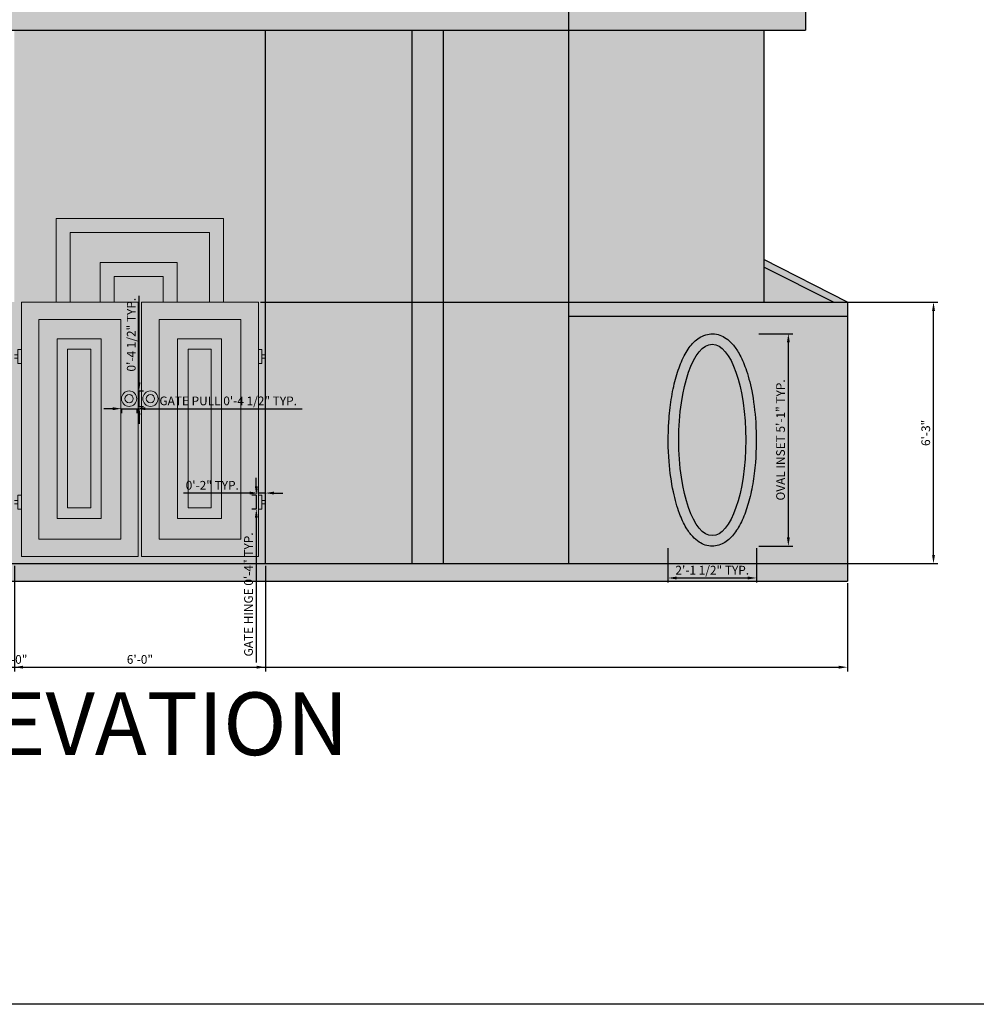
# Model space of a CAD drawing. Units: inches. Extents: x 2169 to 10664, y 1669 to 6352.
# Tile 14 of 17: x 9778 to 10052, y 5159 to 5441. Entities that reach past the tile are written whole.
import ezdxf

# ---------------------------------------------------------------- set-up
doc = ezdxf.new("R2010")
doc.units = ezdxf.units.IN
for name, color, linetype, lineweight in [('A-ANNO-DIMS', 3, 'Continuous', 18), ('A-ANNO-TITL', 3, 'Continuous', 25), ('A-ANNO-TTLB', 7, 'Continuous', 25), ('A-ELEV', 7, 'Continuous', 25), ('A-ELEV-CONC-PATT', 85, 'Continuous', 13), ('A-ELEV-GATE', 7, 'Continuous', 18), ('A-ELEV-GATE-PATT', 252, 'Continuous', 13), ('A-ELEV-OPEN', 7, 'Continuous', 18), ('A-ELEV-OPEN-PATT', 9, 'Continuous', 13), ('A-ELEV-PATT', 253, 'Continuous', 13)]:
    doc.layers.add(name, color=color, linetype=linetype, lineweight=lineweight)
doc.styles.get("Standard").update_dxf_attribs({"font": 'arial.ttf'})
doc.dimstyles.new('ISO-25', dxfattribs={"dimtxt": 2.5, "dimasz": 2.5, "dimexe": 1.25, "dimexo": 0.625, "dimtad": 1, "dimdec": 0, "dimlunit": 3, "dimtxsty": 'Standard', "dimcen": 2.5, "dimadec": 0, "dimazin": 0, "dimtfac": 1, "dimtdec": 0, "dimtmove": 0, "dimatfit": 3, "dimfxl": 1, "dimarcsym": 0})

# ---------------------------------------------------------------- blocks, each defined once
blk = doc.blocks.new('GATE-HINGE-3')
for p, q in [((2, 4), (1, 4)), ((1, 4), (1, 0)), ((1, 2.5), (0, 2.5)), ((1, 1.5), (0, 1.5)), ((2, 0), (1, 0))]:
    blk.add_line(p, q)
blk = doc.blocks.new('GATE-PULL-ROUND')
for radius in [2.2, 1.2]:
    blk.add_circle((2.21, 2.21), radius)
blk = doc.blocks.new('FACADE-OVAL-INSET')
blk.add_ellipse((12.63, 30.44), major_axis=(0, -27.44), ratio=0.350877)
blk.add_open_spline([(12.63, 0), (13.28, 0), (13.93, 0.1), (15.16, 0.48), (15.73, 0.75), (16.8, 1.42), (17.29, 1.81), (18.2, 2.68), (18.63, 3.16), (19.86, 4.78), (20.59, 6.05), (21.9, 8.93), (22.47, 10.53), (23.47, 14), (23.89, 15.87), (24.57, 19.81), (24.82, 21.88), (25.3, 27.78), (25.34, 31.73), (24.89, 38.68), (24.51, 41.73), (23.49, 46.87), (22.91, 49.03), (21.66, 52.55), (21.03, 53.98), (19.74, 56.25), (19.12, 57.16), (17.87, 58.57), (17.27, 59.12), (16.05, 59.96), (15.45, 60.28), (14.17, 60.73), (13.48, 60.86), (12.09, 60.9), (11.4, 60.8), (10.08, 60.4), (9.47, 60.11), (8.34, 59.39), (7.83, 58.96), (6.87, 58.01), (6.43, 57.49), (5.17, 55.76), (4.44, 54.41), (3.14, 51.39), (2.57, 49.71), (1.59, 46.07), (1.19, 44.12), (0.55, 40.02), (0.31, 37.87), (-0.08, 31.9), (-0.06, 28), (0.48, 21.2), (0.89, 18.26), (1.95, 13.31), (2.54, 11.23), (3.8, 7.86), (4.43, 6.5), (5.71, 4.33), (6.34, 3.47), (7.58, 2.13), (8.18, 1.61), (9.39, 0.82), (9.99, 0.52), (11.27, 0.11), (11.95, 0), (12.63, 0)], degree=3, knots=[0, 0, 0, 0, 0.107478, 0.107478, 0.214955, 0.214955, 0.322433, 0.322433, 0.429911, 0.429911, 0.658113, 0.658113, 0.886316, 0.886316, 1.114519, 1.114519, 1.342721, 1.342721, 1.750863, 1.750863, 2.0857, 2.0857, 2.362812, 2.362812, 2.586848, 2.586848, 2.764909, 2.764909, 2.903641, 2.903641, 3.018249, 3.018249, 3.132858, 3.132858, 3.247466, 3.247466, 3.362074, 3.362074, 3.476683, 3.476683, 3.591291, 3.591291, 3.82536, 3.82536, 4.059428, 4.059428, 4.293497, 4.293497, 4.527566, 4.527566, 4.931556, 4.931556, 5.258929, 5.258929, 5.530471, 5.530471, 5.749212, 5.749212, 5.922827, 5.922827, 6.058126, 6.058126, 6.171203, 6.171203, 6.283185, 6.283185, 6.283185, 6.283185])
blk = doc.blocks.new('*D67')
at = {"layer": 'A-ANNO-DIMS', "color": 0, "lineweight": -2, "transparency": 16777216}
for p, q in [((9804.65, 5329.75), (9802.15, 5329.75)), ((9807.15, 5329.78), (9807.15, 5328.5)), ((9807.15, 5329.75), (9811.56, 5329.75)), ((9811.56, 5329.78), (9811.56, 5328.5)), ((9814.06, 5329.75), (9859.02, 5329.75))]:
    blk.add_line(p, q, dxfattribs=at)
at = {"layer": 'A-ANNO-DIMS', "color": 0, "transparency": 16777216}
for points in [[(9804.65, 5330.16), (9804.65, 5329.33), (9807.15, 5329.75)], [(9814.06, 5330.16), (9814.06, 5329.33), (9811.56, 5329.75)]]:
    blk.add_solid(points, dxfattribs=at)
at = {"layer": 'Defpoints', "color": 0, "transparency": 16777216}
for p in [(9807.15, 5330.41), (9811.56, 5330.41), (9811.56, 5329.75)]:
    blk.add_point(p, dxfattribs=at)
at = {"layer": 'A-ANNO-DIMS', "color": 0, "transparency": 16777216, "insert": (9837.79, 5331.66), "char_height": 2.5, "attachment_point": 5}
blk.add_mtext('GATE PULL 0\'-4 1/2" TYP.', dxfattribs=at)
blk = doc.blocks.new('*D68')
at = {"layer": 'A-ANNO-DIMS', "color": 0, "lineweight": -2, "transparency": 16777216}
for p, q in [((9812.22, 5337.32), (9812.22, 5362.13)), ((9812.18, 5334.82), (9813.47, 5334.82)), ((9812.22, 5330.41), (9812.22, 5334.82)), ((9812.18, 5330.41), (9813.47, 5330.41)), ((9812.22, 5327.91), (9812.22, 5325.41))]:
    blk.add_line(p, q, dxfattribs=at)
at = {"layer": 'A-ANNO-DIMS', "color": 0, "transparency": 16777216}
for points in [[(9811.8, 5337.32), (9812.63, 5337.32), (9812.22, 5334.82)], [(9811.8, 5327.91), (9812.63, 5327.91), (9812.22, 5330.41)]]:
    blk.add_solid(points, dxfattribs=at)
at = {"layer": 'Defpoints', "color": 0, "transparency": 16777216}
for p in [(9811.56, 5334.82), (9812.22, 5334.82), (9811.56, 5330.41)]:
    blk.add_point(p, dxfattribs=at)
at = {"layer": 'A-ANNO-DIMS', "color": 0, "transparency": 16777216, "insert": (9810.3, 5350.97), "char_height": 2.5, "attachment_point": 5, "rotation": 90}
blk.add_mtext('0\'-4 1/2" TYP.', dxfattribs=at)
blk = doc.blocks.new('*D71')
at = {"layer": 'A-ANNO-DIMS', "color": 0, "lineweight": -2, "transparency": 16777216}
for p, q in [((9845.86, 5307.45), (9845.86, 5309.95)), ((9845.84, 5304.95), (9844.61, 5304.95)), ((9845.86, 5304.95), (9845.86, 5300.95)), ((9845.84, 5300.95), (9844.61, 5300.95)), ((9845.86, 5298.45), (9845.86, 5256.99))]:
    blk.add_line(p, q, dxfattribs=at)
at = {"layer": 'A-ANNO-DIMS', "color": 0, "transparency": 16777216}
for points in [[(9845.45, 5307.45), (9846.28, 5307.45), (9845.86, 5304.95)], [(9845.45, 5298.45), (9846.28, 5298.45), (9845.86, 5300.95)]]:
    blk.add_solid(points, dxfattribs=at)
at = {"layer": 'Defpoints', "color": 0, "transparency": 16777216}
for p in [(9846.46, 5304.95), (9845.86, 5300.95), (9846.46, 5300.95)]:
    blk.add_point(p, dxfattribs=at)
at = {"layer": 'A-ANNO-DIMS', "color": 0, "transparency": 16777216, "insert": (9843.94, 5276.47), "char_height": 2.5, "attachment_point": 5, "rotation": 90}
blk.add_mtext('GATE HINGE 0\'-4" TYP.', dxfattribs=at)
blk = doc.blocks.new('*D72')
at = {"layer": 'A-ANNO-DIMS', "color": 0, "lineweight": -2, "transparency": 16777216}
for p, q in [((9846.46, 5305.57), (9846.46, 5306.8)), ((9848.46, 5305.57), (9848.46, 5306.8)), ((9843.96, 5305.55), (9824.97, 5305.55)), ((9848.46, 5305.55), (9846.46, 5305.55)), ((9850.96, 5305.55), (9853.46, 5305.55))]:
    blk.add_line(p, q, dxfattribs=at)
at = {"layer": 'A-ANNO-DIMS', "color": 0, "transparency": 16777216}
for points in [[(9843.96, 5305.97), (9843.96, 5305.13), (9846.46, 5305.55)], [(9850.96, 5305.97), (9850.96, 5305.13), (9848.46, 5305.55)]]:
    blk.add_solid(points, dxfattribs=at)
at = {"layer": 'Defpoints', "color": 0, "transparency": 16777216}
for p in [(9846.46, 5305.55), (9846.46, 5304.95), (9848.46, 5304.95)]:
    blk.add_point(p, dxfattribs=at)
at = {"layer": 'A-ANNO-DIMS', "color": 0, "transparency": 16777216, "insert": (9833.22, 5307.45), "char_height": 2.5, "attachment_point": 5}
blk.add_mtext('0\'-2" TYP.', dxfattribs=at)
blk = doc.blocks.new('*D73')
at = {"layer": 'A-ANNO-DIMS', "color": 0, "lineweight": -2, "transparency": 16777216}
for p, q in [((9990.01, 5351.23), (9999.77, 5351.23)), ((9998.52, 5292.83), (9998.52, 5348.73)), ((9990.01, 5290.33), (9999.77, 5290.33))]:
    blk.add_line(p, q, dxfattribs=at)
at = {"layer": 'A-ANNO-DIMS', "color": 0, "transparency": 16777216}
for points in [[(9998.1, 5348.73), (9998.94, 5348.73), (9998.52, 5351.23)], [(9998.1, 5292.83), (9998.94, 5292.83), (9998.52, 5290.33)]]:
    blk.add_solid(points, dxfattribs=at)
at = {"layer": 'Defpoints', "color": 0, "transparency": 16777216}
for p in [(9989.38, 5351.23), (9998.52, 5351.23), (9989.38, 5290.33)]:
    blk.add_point(p, dxfattribs=at)
at = {"layer": 'A-ANNO-DIMS', "color": 0, "transparency": 16777216, "insert": (9996.6, 5320.78), "char_height": 2.5, "attachment_point": 5, "rotation": 90}
blk.add_mtext('OVAL INSET 5\'-1" TYP.', dxfattribs=at)
blk = doc.blocks.new('*D74')
at = {"layer": 'A-ANNO-DIMS', "color": 0, "lineweight": -2, "transparency": 16777216}
for p, q in [((9963.97, 5289.7), (9963.97, 5279.94)), ((9989.38, 5289.7), (9989.38, 5279.94)), ((9966.47, 5281.19), (9986.88, 5281.19))]:
    blk.add_line(p, q, dxfattribs=at)
at = {"layer": 'A-ANNO-DIMS', "color": 0, "transparency": 16777216}
for points in [[(9966.47, 5281.61), (9966.47, 5280.78), (9963.97, 5281.19)], [(9986.88, 5281.61), (9986.88, 5280.78), (9989.38, 5281.19)]]:
    blk.add_solid(points, dxfattribs=at)
at = {"layer": 'Defpoints', "color": 0, "transparency": 16777216}
for p in [(9963.97, 5290.33), (9989.38, 5290.33), (9989.38, 5281.19)]:
    blk.add_point(p, dxfattribs=at)
at = {"layer": 'A-ANNO-DIMS', "color": 0, "transparency": 16777216, "insert": (9976.68, 5283.11), "char_height": 2.5, "attachment_point": 5}
blk.add_mtext('2\'-1 1/2" TYP.', dxfattribs=at)
blk = doc.blocks.new('*D117')
at = {"layer": 'A-ANNO-DIMS', "color": 0, "lineweight": -2, "transparency": 16777216}
for p, q in [((9535.46, 5279.69), (9535.46, 5254.36)), ((10015.46, 5279.69), (10015.46, 5254.36)), ((9537.96, 5255.61), (10012.96, 5255.61))]:
    blk.add_line(p, q, dxfattribs=at)
at = {"layer": 'A-ANNO-DIMS', "color": 0, "transparency": 16777216}
for points in [[(9537.96, 5256.03), (9537.96, 5255.19), (9535.46, 5255.61)], [(10012.96, 5256.03), (10012.96, 5255.19), (10015.46, 5255.61)]]:
    blk.add_solid(points, dxfattribs=at)
at = {"layer": 'Defpoints', "color": 0, "transparency": 16777216}
for p in [(9535.46, 5280.31), (10015.46, 5280.31), (10015.46, 5255.61)]:
    blk.add_point(p, dxfattribs=at)
at = {"layer": 'A-ANNO-DIMS', "color": 0, "transparency": 16777216, "insert": (9775.46, 5257.51), "char_height": 2.5, "attachment_point": 5}
blk.add_mtext('40\'-0"', dxfattribs=at)
blk = doc.blocks.new('*D124')
at = {"layer": 'A-ANNO-DIMS', "color": 0, "lineweight": -2, "transparency": 16777216}
for p, q in [((9776.46, 5284.69), (9776.46, 5254.36)), ((9848.46, 5284.69), (9848.46, 5254.36)), ((9778.96, 5255.61), (9845.96, 5255.61))]:
    blk.add_line(p, q, dxfattribs=at)
at = {"layer": 'A-ANNO-DIMS', "color": 0, "transparency": 16777216}
for points in [[(9778.96, 5256.03), (9778.96, 5255.19), (9776.46, 5255.61)], [(9845.96, 5256.03), (9845.96, 5255.19), (9848.46, 5255.61)]]:
    blk.add_solid(points, dxfattribs=at)
at = {"layer": 'Defpoints', "color": 0, "transparency": 16777216}
for p in [(9776.46, 5285.31), (9848.46, 5285.31), (9848.46, 5255.61)]:
    blk.add_point(p, dxfattribs=at)
at = {"layer": 'A-ANNO-DIMS', "color": 0, "transparency": 16777216, "insert": (9812.46, 5257.51), "char_height": 2.5, "attachment_point": 5}
blk.add_mtext('6\'-0"', dxfattribs=at)
blk = doc.blocks.new('*D125')
at = {"layer": 'A-ANNO-DIMS', "color": 0, "lineweight": -2, "transparency": 16777216}
for p, q in [((9847.09, 5360.31), (10041.41, 5360.31)), ((10040.16, 5287.81), (10040.16, 5357.81)), ((9849.09, 5285.31), (10041.41, 5285.31))]:
    blk.add_line(p, q, dxfattribs=at)
at = {"layer": 'A-ANNO-DIMS', "color": 0, "transparency": 16777216}
for points in [[(10039.75, 5357.81), (10040.58, 5357.81), (10040.16, 5360.31)], [(10039.75, 5287.81), (10040.58, 5287.81), (10040.16, 5285.31)]]:
    blk.add_solid(points, dxfattribs=at)
at = {"layer": 'Defpoints', "color": 0, "transparency": 16777216}
for p in [(9846.46, 5360.31), (10040.16, 5360.31), (9848.46, 5285.31)]:
    blk.add_point(p, dxfattribs=at)
at = {"layer": 'A-ANNO-DIMS', "color": 0, "transparency": 16777216, "insert": (10038.26, 5322.81), "char_height": 2.5, "attachment_point": 5, "rotation": 90}
blk.add_mtext('6\'-3"', dxfattribs=at)

msp = doc.modelspace()

# ---------------------------------------------------------------- hatches: boundary and pattern name
at = {"layer": 'A-ELEV-CONC-PATT'}
h = msp.add_hatch(dxfattribs=at)
h.set_pattern_fill('AR-CONC', color=256, scale=0.02)
h.paths.add_polyline_path([(9899.46, 5522.31), (9776.46, 5522.31), (9776.46, 5513.31), (9890.46, 5513.31), (9890.46, 5444.31), (9899.46, 5444.31)])
h.paths.add_polyline_path([(9899.46, 5438.31), (9890.46, 5438.31), (9890.46, 5285.31), (9899.46, 5285.31)])
at = {"layer": 'A-ELEV-GATE-PATT'}
h = msp.add_hatch(color=256, dxfattribs=at)
h.dxf.hatch_style = 1
h.paths.add_polyline_path([(9778.46, 5346.71), (9777.46, 5346.71), (9777.46, 5342.71), (9778.46, 5342.71)])
h.paths.add_polyline_path([(9777.46, 5345.21), (9776.46, 5345.21), (9776.46, 5344.21), (9777.46, 5344.21)])
h.paths.add_polyline_path([(9848.46, 5345.21), (9847.46, 5345.21), (9847.46, 5344.21), (9848.46, 5344.21)])
h.paths.add_polyline_path([(9847.46, 5346.71), (9846.46, 5346.71), (9846.46, 5342.71), (9847.46, 5342.71)])
h.paths.add_polyline_path([(9847.46, 5304.95), (9846.46, 5304.95), (9846.46, 5300.95), (9847.46, 5300.95)])
h.paths.add_polyline_path([(9848.46, 5303.45), (9847.46, 5303.45), (9847.46, 5302.45), (9848.46, 5302.45)])
h.paths.add_polyline_path([(9778.46, 5304.95), (9777.46, 5304.95), (9777.46, 5300.95), (9778.46, 5300.95)])
h.paths.add_polyline_path([(9777.46, 5303.45), (9776.46, 5303.45), (9776.46, 5302.45), (9777.46, 5302.45)])
h.paths.add_polyline_path([(9811.96, 5360.31), (9778.46, 5360.31), (9778.46, 5287.31), (9811.96, 5287.31)])
h.paths.add_polyline_path([(9783.46, 5355.31), (9806.96, 5355.31), (9806.96, 5292.31), (9783.46, 5292.31)], flags=16)
h.paths.add_polyline_path([(9788.71, 5349.82), (9801.33, 5349.82), (9801.33, 5298.27), (9788.71, 5298.27)], flags=0)
h.paths.add_polyline_path([(9791.71, 5346.82), (9798.33, 5346.82), (9798.33, 5301.27), (9791.71, 5301.27)], flags=0)
h.paths.add_polyline_path([(9807.16, 5332.61, -1), (9811.54, 5332.61, -1)], flags=16)
h.paths.add_polyline_path([(9808.16, 5332.61, -1), (9810.54, 5332.61, -1)], flags=0)
h.paths.add_polyline_path([(9846.46, 5360.31), (9812.96, 5360.31), (9812.96, 5287.31), (9846.46, 5287.31)])
h.paths.add_polyline_path([(9817.96, 5355.31), (9841.46, 5355.31), (9841.46, 5292.31), (9817.96, 5292.31)], flags=16)
h.paths.add_polyline_path([(9823.29, 5349.82), (9835.91, 5349.82), (9835.91, 5298.27), (9823.29, 5298.27)], flags=0)
h.paths.add_polyline_path([(9826.29, 5346.82), (9832.91, 5346.82), (9832.91, 5301.27), (9826.29, 5301.27)], flags=0)
h.paths.add_polyline_path([(9813.3, 5332.61, -1), (9817.67, 5332.61, -1)], flags=16)
h.paths.add_polyline_path([(9814.3, 5332.61, -1), (9816.67, 5332.61, -1)], flags=0)
h.paths.add_polyline_path([(9801.33, 5349.82), (9788.71, 5349.82), (9788.71, 5298.27), (9801.33, 5298.27)], flags=0)
h = msp.add_hatch(color=256, dxfattribs=at)
h.dxf.hatch_style = 1
h.paths.add_polyline_path([(9806.96, 5355.31), (9783.46, 5355.31), (9783.46, 5292.31), (9806.96, 5292.31)])
h.paths.add_polyline_path([(9788.71, 5349.82), (9801.33, 5349.82), (9801.33, 5298.27), (9788.71, 5298.27)], flags=16)
h.paths.add_polyline_path([(9791.71, 5346.82), (9798.33, 5346.82), (9798.33, 5301.27), (9791.71, 5301.27)], flags=0)
h.paths.add_polyline_path([(9841.46, 5355.31), (9817.96, 5355.31), (9817.96, 5292.31), (9841.46, 5292.31)])
h.paths.add_polyline_path([(9823.29, 5349.82), (9835.91, 5349.82), (9835.91, 5298.27), (9823.29, 5298.27)], flags=16)
h.paths.add_polyline_path([(9826.29, 5346.82), (9832.91, 5346.82), (9832.91, 5301.27), (9826.29, 5301.27)], flags=0)
h = msp.add_hatch(color=256, dxfattribs=at)
h.dxf.hatch_style = 1
h.paths.add_polyline_path([(9801.33, 5349.82), (9788.71, 5349.82), (9788.71, 5298.27), (9801.33, 5298.27)])
h.paths.add_polyline_path([(9791.71, 5346.82), (9798.33, 5346.82), (9798.33, 5301.27), (9791.71, 5301.27)], flags=16)
h.paths.add_polyline_path([(9835.91, 5349.82), (9823.29, 5349.82), (9823.29, 5298.27), (9835.91, 5298.27)])
h.paths.add_polyline_path([(9826.29, 5346.82), (9832.91, 5346.82), (9832.91, 5301.27), (9826.29, 5301.27)], flags=16)
h = msp.add_hatch(color=256, dxfattribs=at)
h.dxf.hatch_style = 1
h.paths.add_polyline_path([(9798.33, 5346.82), (9791.71, 5346.82), (9791.71, 5301.27), (9798.33, 5301.27)])
h.paths.add_polyline_path([(9832.91, 5346.82), (9826.29, 5346.82), (9826.29, 5301.27), (9832.91, 5301.27)])
h = msp.add_hatch(color=256, dxfattribs=at)
h.dxf.hatch_style = 1
h.paths.add_polyline_path([(9811.54, 5332.61, 1), (9807.16, 5332.61, 1)])
h.paths.add_polyline_path([(9808.16, 5332.61, -1), (9810.54, 5332.61, -1)], flags=16)
h.paths.add_polyline_path([(9817.67, 5332.61, 1), (9813.3, 5332.61, 1)])
h.paths.add_polyline_path([(9814.3, 5332.61, -1), (9816.67, 5332.61, -1)], flags=16)
h = msp.add_hatch(color=256, dxfattribs=at)
h.dxf.hatch_style = 1
h.paths.add_polyline_path([(9808.16, 5332.61, 1), (9810.54, 5332.61, 1)])
h.paths.add_polyline_path([(9814.3, 5332.61, 1), (9816.67, 5332.61, 1)])
at = {"layer": 'A-ELEV-OPEN-PATT'}
h = msp.add_hatch(color=256, dxfattribs=at)
h.dxf.hatch_style = 1
h.paths.add_polyline_path([(9836.46, 5384.31), (9788.46, 5384.31), (9788.46, 5360.31), (9792.46, 5360.31), (9792.46, 5380.31), (9832.46, 5380.31), (9832.46, 5360.31), (9836.46, 5360.31)])
h.paths.add_polyline_path([(9823.12, 5371.65), (9801.1, 5371.65), (9801.1, 5360.31), (9805.1, 5360.31), (9805.1, 5367.65), (9819.12, 5367.65), (9819.12, 5360.31), (9823.12, 5360.31)], flags=17)
h.paths.add_polyline_path([(9640.46, 5384.31), (9592.46, 5384.31), (9592.46, 5360.31), (9596.46, 5360.31), (9596.46, 5380.31), (9636.46, 5380.31), (9636.46, 5360.31), (9640.46, 5360.31)])
h.paths.add_polyline_path([(9627.69, 5371.73), (9604, 5371.73), (9604, 5360.31), (9608, 5360.31), (9608, 5367.73), (9623.69, 5367.73), (9623.69, 5360.31), (9627.69, 5360.31)], flags=17)
h = msp.add_hatch(color=256, dxfattribs=at)
h.dxf.hatch_style = 1
h.paths.add_polyline_path([(9636.46, 5380.31), (9596.46, 5380.31), (9596.46, 5360.31), (9604, 5360.31), (9604, 5371.73), (9627.69, 5371.73), (9627.69, 5360.31), (9636.46, 5360.31)])
h.paths.add_polyline_path([(9623.69, 5367.73), (9608, 5367.73), (9608, 5360.31), (9623.69, 5360.31)], flags=17)
h.paths.add_polyline_path([(9832.46, 5380.31), (9792.46, 5380.31), (9792.46, 5360.31), (9801.1, 5360.31), (9801.1, 5371.65), (9823.12, 5371.65), (9823.12, 5360.31), (9832.46, 5360.31)])
at = {"layer": 'A-ELEV-PATT'}
h = msp.add_hatch(color=256, dxfattribs=at)
h.dxf.hatch_style = 1
h.paths.add_polyline_path([(10003.46, 5552.31), (9547.46, 5552.31), (9547.46, 5546.31), (10003.46, 5546.31)])
h.paths.add_polyline_path([(9776.46, 5444.31), (9547.46, 5444.31), (9547.46, 5438.31), (9776.46, 5438.31)])
h.paths.add_polyline_path([(9935.46, 5444.31), (9776.46, 5444.31), (9776.46, 5438.31), (9935.46, 5438.31)])
h.paths.add_polyline_path([(10003.46, 5444.31), (9935.46, 5444.31), (9935.46, 5438.31), (10003.46, 5438.31)])
h = msp.add_hatch(color=256, dxfattribs=at)
h.dxf.hatch_style = 1
h.paths.add_polyline_path([(9935.46, 5546.31), (9776.46, 5546.31), (9776.46, 5522.31), (9899.46, 5522.31), (9899.46, 5444.31), (9935.46, 5444.31)])
h.paths.add_polyline_path([(9935.46, 5438.31), (9899.46, 5438.31), (9899.46, 5285.31), (9935.46, 5285.31)])
h.paths.add_polyline_path([(9890.46, 5438.31), (9848.46, 5438.31), (9848.46, 5285.31), (9890.46, 5285.31)])
h.paths.add_polyline_path([(9890.46, 5513.31), (9776.46, 5513.31), (9776.46, 5444.31), (9890.46, 5444.31)], flags=17)
h = msp.add_hatch(color=256, dxfattribs=at)
h.dxf.hatch_style = 1
h.paths.add_polyline_path([(9991.46, 5438.31), (9935.46, 5438.31), (9935.46, 5360.31), (9991.46, 5360.31)])
h.paths.add_polyline_path([(9991.46, 5546.31), (9935.46, 5546.31), (9935.46, 5444.31), (9991.46, 5444.31)])
h = msp.add_hatch(color=256, dxfattribs=at)
h.dxf.hatch_style = 1
h.paths.add_polyline_path([(9848.46, 5438.31), (9776.46, 5438.31), (9776.46, 5345.21), (9777.46, 5345.21), (9777.46, 5346.71), (9778.46, 5346.71), (9778.46, 5360.31), (9788.46, 5360.31), (9788.46, 5384.31), (9836.46, 5384.31), (9836.46, 5360.31), (9846.46, 5360.31), (9846.46, 5346.71), (9847.46, 5346.71), (9847.46, 5345.21), (9848.46, 5345.21)])
h = msp.add_hatch(color=256, dxfattribs=at)
h.dxf.hatch_style = 1
h.paths.add_polyline_path([(9776.46, 5360.31), (9539.46, 5360.31), (9559.46, 5369.86), (9559.46, 5371.85), (9535.46, 5360.31), (9535.46, 5356.31), (9776.46, 5356.31)])
h.paths.add_polyline_path([(10015.46, 5360.31), (9991.46, 5372.52), (9991.46, 5370.33), (10011.46, 5360.31), (9935.46, 5360.31), (9935.46, 5356.31), (10015.46, 5356.31)])
h = msp.add_hatch(color=256, dxfattribs=at)
h.dxf.hatch_style = 1
h.paths.add_polyline_path([(9559.46, 5369.86), (9539.46, 5360.31), (9559.46, 5360.31)])
h.paths.add_polyline_path([(9991.46, 5370.33), (9991.46, 5360.31), (10011.46, 5360.31)])
h = msp.add_hatch(color=256, dxfattribs=at)
h.dxf.hatch_style = 1
h.paths.add_polyline_path([(9778.46, 5342.71), (9777.46, 5342.71), (9777.46, 5344.21), (9776.46, 5344.21), (9776.46, 5303.45), (9777.46, 5303.45), (9777.46, 5304.95), (9778.46, 5304.95)], flags=17)
h.paths.add_polyline_path([(9848.46, 5344.21), (9847.46, 5344.21), (9847.46, 5342.71), (9846.46, 5342.71), (9846.46, 5304.95), (9847.46, 5304.95), (9847.46, 5303.45), (9848.46, 5303.45)], flags=17)
h.paths.add_polyline_path([(9778.46, 5300.95), (9777.46, 5300.95), (9777.46, 5302.45), (9776.46, 5302.45), (9776.46, 5285.31), (9848.46, 5285.31), (9848.46, 5302.45), (9847.46, 5302.45), (9847.46, 5300.95), (9846.46, 5300.95), (9846.46, 5287.31), (9812.96, 5287.31), (9812.96, 5360.31), (9819.12, 5360.31), (9819.12, 5367.65), (9805.1, 5367.65), (9805.1, 5360.31), (9811.96, 5360.31), (9811.96, 5287.31), (9778.46, 5287.31)])
h = msp.add_hatch(color=256, dxfattribs=at)
h.dxf.hatch_style = 1
h.paths.add_polyline_path([(9776.46, 5356.31), (9535.46, 5356.31), (9535.46, 5285.31), (9776.46, 5285.31)])
edge = h.paths.add_edge_path(flags=16)
edge.add_spline(control_points=[(9649.63, 5290.33), (9650.28, 5290.33), (9650.93, 5290.43), (9652.16, 5290.81), (9652.74, 5291.08), (9653.8, 5291.75), (9654.29, 5292.14), (9655.21, 5293.01), (9655.63, 5293.48), (9656.87, 5295.1), (9657.6, 5296.38), (9658.9, 5299.26), (9659.48, 5300.86), (9660.47, 5304.33), (9660.89, 5306.2), (9661.57, 5310.14), (9661.83, 5312.21), (9662.31, 5318.11), (9662.34, 5322.06), (9661.9, 5329.01), (9661.51, 5332.06), (9660.49, 5337.2), (9659.91, 5339.36), (9658.66, 5342.88), (9658.03, 5344.31), (9656.74, 5346.58), (9656.12, 5347.49), (9654.87, 5348.9), (9654.27, 5349.45), (9653.06, 5350.29), (9652.46, 5350.61), (9651.17, 5351.06), (9650.48, 5351.19), (9649.1, 5351.23), (9648.4, 5351.13), (9647.09, 5350.73), (9646.47, 5350.44), (9645.35, 5349.72), (9644.83, 5349.29), (9643.87, 5348.34), (9643.43, 5347.82), (9642.18, 5346.09), (9641.44, 5344.74), (9640.14, 5341.72), (9639.57, 5340.04), (9638.6, 5336.4), (9638.19, 5334.45), (9637.55, 5330.34), (9637.32, 5328.2), (9636.93, 5322.23), (9636.95, 5318.33), (9637.48, 5311.53), (9637.89, 5308.59), (9638.95, 5303.64), (9639.54, 5301.56), (9640.8, 5298.19), (9641.43, 5296.83), (9642.72, 5294.66), (9643.34, 5293.8), (9644.59, 5292.46), (9645.18, 5291.94), (9646.4, 5291.15), (9647, 5290.85), (9648.28, 5290.44), (9648.95, 5290.33), (9649.63, 5290.33)], knot_values=[0, 0, 0, 0, 0.107478, 0.107478, 0.214955, 0.214955, 0.322433, 0.322433, 0.429911, 0.429911, 0.658113, 0.658113, 0.886316, 0.886316, 1.114519, 1.114519, 1.342721, 1.342721, 1.750863, 1.750863, 2.0857, 2.0857, 2.362812, 2.362812, 2.586848, 2.586848, 2.764909, 2.764909, 2.903641, 2.903641, 3.018249, 3.018249, 3.132858, 3.132858, 3.247466, 3.247466, 3.362074, 3.362074, 3.476683, 3.476683, 3.591291, 3.591291, 3.82536, 3.82536, 4.059428, 4.059428, 4.293497, 4.293497, 4.527566, 4.527566, 4.931556, 4.931556, 5.258929, 5.258929, 5.530471, 5.530471, 5.749212, 5.749212, 5.922827, 5.922827, 6.058126, 6.058126, 6.171203, 6.171203, 6.283185, 6.283185, 6.283185, 6.283185], degree=3, periodic=0)
edge = h.paths.add_edge_path(flags=16)
edge.add_spline(control_points=[(9575.48, 5290.33), (9576.13, 5290.33), (9576.78, 5290.43), (9578.01, 5290.81), (9578.59, 5291.08), (9579.65, 5291.75), (9580.15, 5292.14), (9581.06, 5293.01), (9581.48, 5293.48), (9582.72, 5295.1), (9583.45, 5296.38), (9584.76, 5299.26), (9585.33, 5300.86), (9586.32, 5304.33), (9586.74, 5306.2), (9587.42, 5310.14), (9587.68, 5312.21), (9588.16, 5318.11), (9588.19, 5322.06), (9587.75, 5329.01), (9587.36, 5332.06), (9586.34, 5337.2), (9585.76, 5339.36), (9584.51, 5342.88), (9583.88, 5344.31), (9582.59, 5346.58), (9581.97, 5347.49), (9580.72, 5348.9), (9580.12, 5349.45), (9578.91, 5350.29), (9578.31, 5350.61), (9577.02, 5351.06), (9576.33, 5351.19), (9574.95, 5351.23), (9574.25, 5351.13), (9572.94, 5350.73), (9572.33, 5350.44), (9571.2, 5349.72), (9570.68, 5349.29), (9569.72, 5348.34), (9569.28, 5347.82), (9568.03, 5346.09), (9567.29, 5344.74), (9565.99, 5341.72), (9565.42, 5340.04), (9564.45, 5336.4), (9564.04, 5334.45), (9563.4, 5330.34), (9563.17, 5328.2), (9562.78, 5322.23), (9562.8, 5318.33), (9563.33, 5311.53), (9563.74, 5308.59), (9564.8, 5303.64), (9565.39, 5301.56), (9566.65, 5298.19), (9567.29, 5296.83), (9568.57, 5294.66), (9569.19, 5293.8), (9570.44, 5292.46), (9571.03, 5291.94), (9572.25, 5291.15), (9572.85, 5290.85), (9574.13, 5290.44), (9574.8, 5290.33), (9575.48, 5290.33)], knot_values=[0, 0, 0, 0, 0.107478, 0.107478, 0.214955, 0.214955, 0.322433, 0.322433, 0.429911, 0.429911, 0.658113, 0.658113, 0.886316, 0.886316, 1.114519, 1.114519, 1.342721, 1.342721, 1.750863, 1.750863, 2.0857, 2.0857, 2.362812, 2.362812, 2.586848, 2.586848, 2.764909, 2.764909, 2.903641, 2.903641, 3.018249, 3.018249, 3.132858, 3.132858, 3.247466, 3.247466, 3.362074, 3.362074, 3.476683, 3.476683, 3.591291, 3.591291, 3.82536, 3.82536, 4.059428, 4.059428, 4.293497, 4.293497, 4.527566, 4.527566, 4.931556, 4.931556, 5.258929, 5.258929, 5.530471, 5.530471, 5.749212, 5.749212, 5.922827, 5.922827, 6.058126, 6.058126, 6.171203, 6.171203, 6.283185, 6.283185, 6.283185, 6.283185], degree=3, periodic=0)
edge = h.paths.add_edge_path(flags=0)
edge.add_ellipse((9649.63, 5320.77), major_axis=(0, -27.44), ratio=0.350877, start_angle=0, end_angle=360)
edge = h.paths.add_edge_path(flags=0)
edge.add_ellipse((9575.48, 5320.77), major_axis=(0, -27.44), ratio=0.350877, start_angle=0, end_angle=360)
edge = h.paths.add_edge_path(flags=16)
edge.add_spline(control_points=[(9728.75, 5290.33), (9729.4, 5290.33), (9730.05, 5290.43), (9731.28, 5290.81), (9731.86, 5291.08), (9732.92, 5291.75), (9733.41, 5292.14), (9734.33, 5293.01), (9734.75, 5293.48), (9735.99, 5295.1), (9736.72, 5296.38), (9738.02, 5299.26), (9738.6, 5300.86), (9739.59, 5304.33), (9740.01, 5306.2), (9740.69, 5310.14), (9740.95, 5312.21), (9741.43, 5318.11), (9741.46, 5322.06), (9741.02, 5329.01), (9740.63, 5332.06), (9739.61, 5337.2), (9739.03, 5339.36), (9737.78, 5342.88), (9737.15, 5344.31), (9735.86, 5346.58), (9735.24, 5347.49), (9733.99, 5348.9), (9733.39, 5349.45), (9732.18, 5350.29), (9731.58, 5350.61), (9730.29, 5351.06), (9729.6, 5351.19), (9728.22, 5351.23), (9727.52, 5351.13), (9726.21, 5350.73), (9725.59, 5350.44), (9724.47, 5349.72), (9723.95, 5349.29), (9722.99, 5348.34), (9722.55, 5347.82), (9721.29, 5346.09), (9720.56, 5344.74), (9719.26, 5341.72), (9718.69, 5340.04), (9717.72, 5336.4), (9717.31, 5334.45), (9716.67, 5330.34), (9716.44, 5328.2), (9716.04, 5322.23), (9716.07, 5318.33), (9716.6, 5311.53), (9717.01, 5308.59), (9718.07, 5303.64), (9718.66, 5301.56), (9719.92, 5298.19), (9720.55, 5296.83), (9721.84, 5294.66), (9722.46, 5293.8), (9723.71, 5292.46), (9724.3, 5291.94), (9725.52, 5291.15), (9726.12, 5290.85), (9727.4, 5290.44), (9728.07, 5290.33), (9728.75, 5290.33)], knot_values=[0, 0, 0, 0, 0.107478, 0.107478, 0.214955, 0.214955, 0.322433, 0.322433, 0.429911, 0.429911, 0.658113, 0.658113, 0.886316, 0.886316, 1.114519, 1.114519, 1.342721, 1.342721, 1.750863, 1.750863, 2.0857, 2.0857, 2.362812, 2.362812, 2.586848, 2.586848, 2.764909, 2.764909, 2.903641, 2.903641, 3.018249, 3.018249, 3.132858, 3.132858, 3.247466, 3.247466, 3.362074, 3.362074, 3.476683, 3.476683, 3.591291, 3.591291, 3.82536, 3.82536, 4.059428, 4.059428, 4.293497, 4.293497, 4.527566, 4.527566, 4.931556, 4.931556, 5.258929, 5.258929, 5.530471, 5.530471, 5.749212, 5.749212, 5.922827, 5.922827, 6.058126, 6.058126, 6.171203, 6.171203, 6.283185, 6.283185, 6.283185, 6.283185], degree=3, periodic=0)
edge = h.paths.add_edge_path(flags=0)
edge.add_ellipse((9728.75, 5320.77), major_axis=(0, -27.44), ratio=0.350877, start_angle=0, end_angle=360)
h.paths.add_polyline_path([(10015.46, 5356.31), (9935.46, 5356.31), (9935.46, 5285.31), (10015.46, 5285.31)])
edge = h.paths.add_edge_path(flags=16)
edge.add_spline(control_points=[(9976.67, 5290.33), (9977.32, 5290.33), (9977.97, 5290.43), (9979.2, 5290.81), (9979.78, 5291.08), (9980.85, 5291.75), (9981.34, 5292.14), (9982.25, 5293.01), (9982.67, 5293.48), (9983.91, 5295.1), (9984.64, 5296.38), (9985.95, 5299.26), (9986.52, 5300.86), (9987.51, 5304.33), (9987.93, 5306.2), (9988.61, 5310.14), (9988.87, 5312.21), (9989.35, 5318.11), (9989.38, 5322.06), (9988.94, 5329.01), (9988.55, 5332.06), (9987.53, 5337.2), (9986.95, 5339.36), (9985.7, 5342.88), (9985.07, 5344.31), (9983.79, 5346.58), (9983.16, 5347.49), (9981.91, 5348.9), (9981.31, 5349.45), (9980.1, 5350.29), (9979.5, 5350.61), (9978.21, 5351.06), (9977.53, 5351.19), (9976.14, 5351.23), (9975.44, 5351.13), (9974.13, 5350.73), (9973.52, 5350.44), (9972.39, 5349.72), (9971.87, 5349.29), (9970.91, 5348.34), (9970.47, 5347.82), (9969.22, 5346.09), (9968.49, 5344.74), (9967.18, 5341.72), (9966.62, 5340.04), (9965.64, 5336.4), (9965.23, 5334.45), (9964.59, 5330.34), (9964.36, 5328.2), (9963.97, 5322.23), (9963.99, 5318.33), (9964.52, 5311.53), (9964.94, 5308.59), (9965.99, 5303.64), (9966.58, 5301.56), (9967.84, 5298.19), (9968.48, 5296.83), (9969.76, 5294.66), (9970.38, 5293.8), (9971.63, 5292.46), (9972.22, 5291.94), (9973.44, 5291.15), (9974.04, 5290.85), (9975.32, 5290.44), (9975.99, 5290.33), (9976.67, 5290.33)], knot_values=[0, 0, 0, 0, 0.107478, 0.107478, 0.214955, 0.214955, 0.322433, 0.322433, 0.429911, 0.429911, 0.658113, 0.658113, 0.886316, 0.886316, 1.114519, 1.114519, 1.342721, 1.342721, 1.750863, 1.750863, 2.0857, 2.0857, 2.362812, 2.362812, 2.586848, 2.586848, 2.764909, 2.764909, 2.903641, 2.903641, 3.018249, 3.018249, 3.132858, 3.132858, 3.247466, 3.247466, 3.362074, 3.362074, 3.476683, 3.476683, 3.591291, 3.591291, 3.82536, 3.82536, 4.059428, 4.059428, 4.293497, 4.293497, 4.527566, 4.527566, 4.931556, 4.931556, 5.258929, 5.258929, 5.530471, 5.530471, 5.749212, 5.749212, 5.922827, 5.922827, 6.058126, 6.058126, 6.171203, 6.171203, 6.283185, 6.283185, 6.283185, 6.283185], degree=3, periodic=0)
edge = h.paths.add_edge_path(flags=0)
edge.add_ellipse((9976.67, 5320.77), major_axis=(0, -27.44), ratio=0.350877, start_angle=0, end_angle=360)
h = msp.add_hatch(color=256, dxfattribs=at)
h.dxf.hatch_style = 1
edge = h.paths.add_edge_path()
edge.add_spline(control_points=[(9976.67, 5290.33), (9977.32, 5290.33), (9977.97, 5290.43), (9979.2, 5290.81), (9979.78, 5291.08), (9980.85, 5291.75), (9981.34, 5292.14), (9982.25, 5293.01), (9982.67, 5293.48), (9983.91, 5295.1), (9984.64, 5296.38), (9985.95, 5299.26), (9986.52, 5300.86), (9987.51, 5304.33), (9987.93, 5306.2), (9988.61, 5310.14), (9988.87, 5312.21), (9989.35, 5318.11), (9989.38, 5322.06), (9988.94, 5329.01), (9988.55, 5332.06), (9987.53, 5337.2), (9986.95, 5339.36), (9985.7, 5342.88), (9985.07, 5344.31), (9983.79, 5346.58), (9983.16, 5347.49), (9981.91, 5348.9), (9981.31, 5349.45), (9980.1, 5350.29), (9979.5, 5350.61), (9978.21, 5351.06), (9977.53, 5351.19), (9976.14, 5351.23), (9975.44, 5351.13), (9974.13, 5350.73), (9973.52, 5350.44), (9972.39, 5349.72), (9971.87, 5349.29), (9970.91, 5348.34), (9970.47, 5347.82), (9969.22, 5346.09), (9968.49, 5344.74), (9967.18, 5341.72), (9966.62, 5340.04), (9965.64, 5336.4), (9965.23, 5334.45), (9964.59, 5330.34), (9964.36, 5328.2), (9963.97, 5322.23), (9963.99, 5318.33), (9964.52, 5311.53), (9964.94, 5308.59), (9965.99, 5303.64), (9966.58, 5301.56), (9967.84, 5298.19), (9968.48, 5296.83), (9969.76, 5294.66), (9970.38, 5293.8), (9971.63, 5292.46), (9972.22, 5291.94), (9973.44, 5291.15), (9974.04, 5290.85), (9975.32, 5290.44), (9975.99, 5290.33), (9976.67, 5290.33)], knot_values=[0, 0, 0, 0, 0.107478, 0.107478, 0.214955, 0.214955, 0.322433, 0.322433, 0.429911, 0.429911, 0.658113, 0.658113, 0.886316, 0.886316, 1.114519, 1.114519, 1.342721, 1.342721, 1.750863, 1.750863, 2.0857, 2.0857, 2.362812, 2.362812, 2.586848, 2.586848, 2.764909, 2.764909, 2.903641, 2.903641, 3.018249, 3.018249, 3.132858, 3.132858, 3.247466, 3.247466, 3.362074, 3.362074, 3.476683, 3.476683, 3.591291, 3.591291, 3.82536, 3.82536, 4.059428, 4.059428, 4.293497, 4.293497, 4.527566, 4.527566, 4.931556, 4.931556, 5.258929, 5.258929, 5.530471, 5.530471, 5.749212, 5.749212, 5.922827, 5.922827, 6.058126, 6.058126, 6.171203, 6.171203, 6.283185, 6.283185, 6.283185, 6.283185], degree=3, periodic=0)
edge = h.paths.add_edge_path(flags=16)
edge.add_ellipse((9976.67, 5320.77), major_axis=(0, -27.44), ratio=0.350877, start_angle=0, end_angle=360)
edge = h.paths.add_edge_path()
edge.add_spline(control_points=[(9728.75, 5290.33), (9729.4, 5290.33), (9730.05, 5290.43), (9731.28, 5290.81), (9731.86, 5291.08), (9732.92, 5291.75), (9733.41, 5292.14), (9734.33, 5293.01), (9734.75, 5293.48), (9735.99, 5295.1), (9736.72, 5296.38), (9738.02, 5299.26), (9738.6, 5300.86), (9739.59, 5304.33), (9740.01, 5306.2), (9740.69, 5310.14), (9740.95, 5312.21), (9741.43, 5318.11), (9741.46, 5322.06), (9741.02, 5329.01), (9740.63, 5332.06), (9739.61, 5337.2), (9739.03, 5339.36), (9737.78, 5342.88), (9737.15, 5344.31), (9735.86, 5346.58), (9735.24, 5347.49), (9733.99, 5348.9), (9733.39, 5349.45), (9732.18, 5350.29), (9731.58, 5350.61), (9730.29, 5351.06), (9729.6, 5351.19), (9728.22, 5351.23), (9727.52, 5351.13), (9726.21, 5350.73), (9725.59, 5350.44), (9724.47, 5349.72), (9723.95, 5349.29), (9722.99, 5348.34), (9722.55, 5347.82), (9721.29, 5346.09), (9720.56, 5344.74), (9719.26, 5341.72), (9718.69, 5340.04), (9717.72, 5336.4), (9717.31, 5334.45), (9716.67, 5330.34), (9716.44, 5328.2), (9716.04, 5322.23), (9716.07, 5318.33), (9716.6, 5311.53), (9717.01, 5308.59), (9718.07, 5303.64), (9718.66, 5301.56), (9719.92, 5298.19), (9720.55, 5296.83), (9721.84, 5294.66), (9722.46, 5293.8), (9723.71, 5292.46), (9724.3, 5291.94), (9725.52, 5291.15), (9726.12, 5290.85), (9727.4, 5290.44), (9728.07, 5290.33), (9728.75, 5290.33)], knot_values=[0, 0, 0, 0, 0.107478, 0.107478, 0.214955, 0.214955, 0.322433, 0.322433, 0.429911, 0.429911, 0.658113, 0.658113, 0.886316, 0.886316, 1.114519, 1.114519, 1.342721, 1.342721, 1.750863, 1.750863, 2.0857, 2.0857, 2.362812, 2.362812, 2.586848, 2.586848, 2.764909, 2.764909, 2.903641, 2.903641, 3.018249, 3.018249, 3.132858, 3.132858, 3.247466, 3.247466, 3.362074, 3.362074, 3.476683, 3.476683, 3.591291, 3.591291, 3.82536, 3.82536, 4.059428, 4.059428, 4.293497, 4.293497, 4.527566, 4.527566, 4.931556, 4.931556, 5.258929, 5.258929, 5.530471, 5.530471, 5.749212, 5.749212, 5.922827, 5.922827, 6.058126, 6.058126, 6.171203, 6.171203, 6.283185, 6.283185, 6.283185, 6.283185], degree=3, periodic=0)
edge = h.paths.add_edge_path(flags=16)
edge.add_ellipse((9728.75, 5320.77), major_axis=(0, -27.44), ratio=0.350877, start_angle=0, end_angle=360)
h = msp.add_hatch(color=256, dxfattribs=at)
h.dxf.hatch_style = 1
edge = h.paths.add_edge_path()
edge.add_ellipse((9575.48, 5320.77), major_axis=(0, -27.44), ratio=0.350877, start_angle=0, end_angle=360)
edge = h.paths.add_edge_path()
edge.add_ellipse((9649.63, 5320.77), major_axis=(0, -27.44), ratio=0.350877, start_angle=0, end_angle=360)
edge = h.paths.add_edge_path()
edge.add_ellipse((9728.75, 5320.77), major_axis=(0, -27.44), ratio=0.350877, start_angle=0, end_angle=360)
edge = h.paths.add_edge_path()
edge.add_ellipse((9976.67, 5320.77), major_axis=(0, -27.44), ratio=0.350877, start_angle=0, end_angle=360)
h = msp.add_hatch(color=256, dxfattribs=at)
h.dxf.hatch_style = 1
h.paths.add_polyline_path([(10015.46, 5285.31), (9535.46, 5285.31), (9535.46, 5280.31), (10015.46, 5280.31)])

# ---------------------------------------------------------------- linework, layer by layer
at = {"layer": 'A-ANNO-TTLB'}
msp.add_lwpolyline([(9414.82, 6351.94), (10664.28, 6351.94), (10664.28, 5158.92), (9414.82, 5158.92)], close=True, dxfattribs=at)
at = {"layer": 'A-ELEV'}
for p, q in [((9935.46, 5546.31), (9935.46, 5285.31)), ((10003.46, 5444.31), (10003.46, 5438.31)), ((9547.46, 5438.31), (9935.46, 5438.31)), ((9848.46, 5285.31), (9848.46, 5438.31)), ((9890.46, 5438.31), (9890.46, 5285.31)), ((9899.46, 5438.31), (9899.46, 5285.31)), ((9935.46, 5438.31), (10003.46, 5438.31)), ((9991.46, 5438.31), (9991.46, 5360.31)), ((10015.46, 5360.31), (9991.46, 5372.52)), ((10011.46, 5360.31), (9991.46, 5370.33)), ((9935.46, 5360.31), (10011.46, 5360.31)), ((10015.46, 5360.31), (10015.46, 5280.31)), ((9935.46, 5356.31), (10015.46, 5356.31)), ((9535.46, 5285.31), (10015.46, 5285.31)), ((9535.46, 5280.31), (10015.46, 5280.31))]:
    msp.add_line(p, q, dxfattribs=at)
at = {"layer": 'A-ELEV-GATE'}
for p, q in [((9778.46, 5360.31), (9778.46, 5287.31)), ((9778.46, 5360.31), (9811.96, 5360.31)), ((9811.96, 5360.31), (9811.96, 5287.31)), ((9812.96, 5360.31), (9812.96, 5287.31)), ((9812.96, 5360.31), (9846.46, 5360.31)), ((9846.46, 5287.31), (9846.46, 5360.31)), ((9783.46, 5355.31), (9783.46, 5292.31)), ((9783.46, 5355.31), (9806.96, 5355.31)), ((9806.96, 5355.31), (9806.96, 5292.31)), ((9817.96, 5355.31), (9841.46, 5355.31)), ((9817.96, 5355.31), (9817.96, 5292.31)), ((9841.46, 5292.31), (9841.46, 5355.31)), ((9783.46, 5292.31), (9806.96, 5292.31)), ((9817.96, 5292.31), (9841.46, 5292.31)), ((9778.46, 5287.31), (9811.96, 5287.31)), ((9812.96, 5287.31), (9846.46, 5287.31))]:
    msp.add_line(p, q, dxfattribs=at)
for points in [[(9788.71, 5349.82), (9801.33, 5349.82), (9801.33, 5298.27), (9788.71, 5298.27)], [(9823.29, 5349.82), (9835.91, 5349.82), (9835.91, 5298.27), (9823.29, 5298.27)], [(9791.71, 5346.82), (9798.33, 5346.82), (9798.33, 5301.27), (9791.71, 5301.27)], [(9826.29, 5346.82), (9832.91, 5346.82), (9832.91, 5301.27), (9826.29, 5301.27)]]:
    msp.add_lwpolyline(points, close=True, dxfattribs=at)
at = {"layer": 'A-ELEV-OPEN'}
for p, q in [((9788.46, 5360.31), (9788.46, 5384.31)), ((9788.46, 5384.31), (9836.46, 5384.31)), ((9836.46, 5360.31), (9836.46, 5384.31)), ((9792.46, 5360.31), (9792.46, 5380.31)), ((9792.46, 5380.31), (9832.46, 5380.31)), ((9832.46, 5360.31), (9832.46, 5380.31))]:
    msp.add_line(p, q, dxfattribs=at)
for points in [[(9801.1, 5360.31), (9801.1, 5371.65), (9823.12, 5371.65), (9823.12, 5360.31)], [(9805.1, 5360.31), (9805.1, 5367.65), (9819.12, 5367.65), (9819.12, 5360.31)]]:
    msp.add_lwpolyline(points, dxfattribs=at)

# ---------------------------------------------------------------- block references
at = {"layer": 'A-ELEV'}
msp.add_blockref('FACADE-OVAL-INSET', (9964.05, 5290.33), dxfattribs=at)
at = {"layer": 'A-ELEV-GATE'}
for name, p in [('GATE-HINGE-3', (9776.46, 5342.71)), ('GATE-PULL-ROUND', (9807.15, 5330.41)), ('GATE-PULL-ROUND', (9813.28, 5330.41)), ('GATE-HINGE-3', (9776.46, 5300.95))]:
    msp.add_blockref(name, p, dxfattribs=at)
at = {"layer": 'A-ELEV-GATE', "rotation": 180}
for p in [(9848.46, 5346.71), (9848.46, 5304.95)]:
    msp.add_blockref('GATE-HINGE-3', p, dxfattribs=at)

# ---------------------------------------------------------------- texts
at = {"layer": 'A-ANNO-TITL', "insert": (9657.79, 5248.39), "char_height": 18, "attachment_point": 1}
msp.add_mtext_dynamic_manual_height_columns('FRONT ELEVATION', width=348.3214, gutter_width=12.5, heights=[0], dxfattribs=at)

# ---------------------------------------------------------------- dimensions: what is measured, and where the dimension line sits
at = {"layer": 'A-ANNO-DIMS'}
for base, p1, p2, angle, text, picture, middle in [((9812.22, 5334.82), (9811.56, 5330.41), (9811.56, 5334.82), 90, '<> TYP.', '*D68', (9810.3, 5350.97)), ((9998.52, 5351.23), (9989.38, 5290.33), (9989.38, 5351.23), 90, 'OVAL INSET <> TYP.', '*D73', (9996.6, 5320.78)), ((9846.46, 5305.55), (9848.46, 5304.95), (9846.46, 5304.95), 180, '<> TYP.', '*D72', (9833.22, 5307.45)), ((9845.86, 5300.95), (9846.46, 5304.95), (9846.46, 5300.95), 270, 'GATE HINGE <> TYP.', '*D71', (9843.94, 5276.47))]:
    dim = msp.add_linear_dim(base=base, p1=p1, p2=p2, angle=angle, text=text, dimstyle='ISO-25', override={"dimdec": 1, "dimlfac": 1, "dimrnd": 0, "dimzin": 1, "dimdsep": 46, "dimlunit": 4, "dimfrac": 2}, dxfattribs=at)
    dim.commit()
    dim.dimension.update_dxf_attribs({"geometry": picture, "text_midpoint": middle})
dim = msp.add_linear_dim(base=(10040.16, 5360.31), p1=(9848.46, 5285.31), p2=(9846.46, 5360.31), angle=90, dimstyle='ISO-25', override={"dimdec": 1, "dimlfac": 1, "dimrnd": 0, "dimzin": 1, "dimdsep": 46, "dimlunit": 4, "dimfrac": 2}, dxfattribs=at)
dim.commit()
dim.dimension.update_dxf_attribs({"geometry": '*D125', "text_midpoint": (10038.26, 5322.81)})
for base, p1, p2, text, picture, middle in [((9811.56, 5329.75), (9807.15, 5330.41), (9811.56, 5330.41), 'GATE PULL <> TYP.', '*D67', (9837.79, 5331.66)), ((9989.38, 5281.19), (9963.97, 5290.33), (9989.38, 5290.33), '<> TYP.', '*D74', (9976.68, 5283.11))]:
    dim = msp.add_linear_dim(base=base, p1=p1, p2=p2, text=text, dimstyle='ISO-25', override={"dimdec": 1, "dimlfac": 1, "dimrnd": 0, "dimzin": 1, "dimdsep": 46, "dimlunit": 4, "dimfrac": 2}, dxfattribs=at)
    dim.commit()
    dim.dimension.update_dxf_attribs({"geometry": picture, "text_midpoint": middle})
for base, p1, p2, picture, middle in [((9848.46, 5255.61), (9776.46, 5285.31), (9848.46, 5285.31), '*D124', (9812.46, 5257.51)), ((10015.46, 5255.61), (9535.46, 5280.31), (10015.46, 5280.31), '*D117', (9775.46, 5257.51))]:
    dim = msp.add_linear_dim(base=base, p1=p1, p2=p2, dimstyle='ISO-25', override={"dimdec": 1, "dimlfac": 1, "dimrnd": 0, "dimzin": 1, "dimdsep": 46, "dimlunit": 4, "dimfrac": 2}, dxfattribs=at)
    dim.commit()
    dim.dimension.update_dxf_attribs({"geometry": picture, "text_midpoint": middle})

doc.saveas('drawing.dxf')
